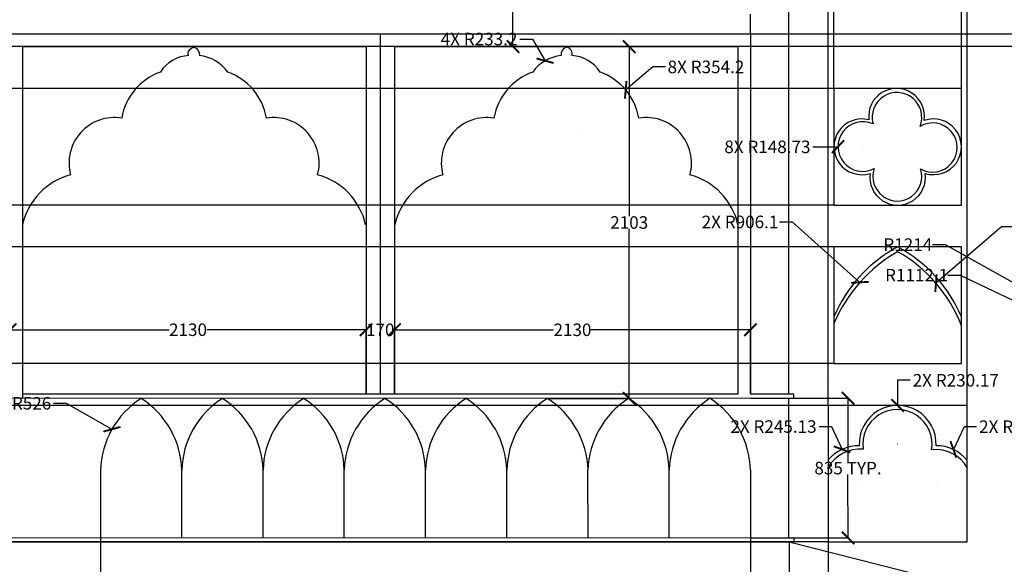
# Model space of a CAD drawing. Units: inches. Extents: x 829 to 33356404, y 1874 to 16983.
# Tile 4 of 9: x 4957 to 10848, y 9032 to 12288. Entities that reach past the tile are written whole.
import ezdxf

# ---------------------------------------------------------------- set-up
doc = ezdxf.new("R2010")
doc.units = ezdxf.units.IN
doc.header["$MEASUREMENT"] = 0
doc.header["$PDMODE"] = 3
doc.layers.add('A-ANNO-DIMS', color=2, linetype='Continuous', lineweight=18)
doc.layers.add('A-ELEV', color=7, linetype='Continuous', lineweight=25)
doc.styles.get("Standard").update_dxf_attribs({"font": 'arial.ttf'})
doc.dimstyles.get("Standard").update_dxf_attribs({"dimtxt": 75, "dimasz": 75, "dimexe": 0.18, "dimexo": 0.0625, "dimgap": 0.09, "dimtad": 0, "dimtih": 1, "dimtoh": 1, "dimdec": 0, "dimzin": 0, "dimdsep": 46, "dimtxsty": 'Standard', "dimblk": 'ARCHTICK', "dimcen": 0.09, "dimadec": 0, "dimazin": 0, "dimtfac": 1, "dimtdec": 0, "dimtofl": 0, "dimtmove": 0, "dimatfit": 3, "dimfxl": 1, "dimtolj": 1, "dimtzin": 0, "dimarcsym": 0})

# ---------------------------------------------------------------- blocks, each defined once
blk = doc.blocks.new('_ArchTick')
at = {"color": 0, "linetype": 'ByBlock', "const_width": 0.15}
blk.add_lwpolyline([(-0.5, -0.5), (0.5, 0.5)], dxfattribs=at)
blk = doc.blocks.new('*D35')
at = {"layer": 'A-ANNO-DIMS', "color": 0, "lineweight": -2, "transparency": 16777216}
for p, q in [((7957.3, 12669.2), (7908.7, 12669.2)), ((7908.8, 12669.2), (7908.8, 12434.2)), ((7908.8, 12127.2), (7908.8, 12357.4)), ((7957.3, 12127.2), (7908.7, 12127.2))]:
    blk.add_line(p, q, dxfattribs=at)
at = {"layer": 'Defpoints', "color": 0, "transparency": 16777216}
for p in [(7908.8, 12669.2), (7957.3, 12669.2), (7957.3, 12127.2)]:
    blk.add_point(p, dxfattribs=at)
at = {"layer": 'A-ANNO-DIMS', "color": 0, "lineweight": -2, "transparency": 16777216, "xscale": 75, "yscale": 75, "zscale": 75}
for p, rotation in [((7908.8, 12669.2), 90), ((7908.8, 12127.2), 270)]:
    blk.add_blockref('_ArchTick', p, dxfattribs=dict(at, rotation=rotation))
at = {"layer": 'A-ANNO-DIMS', "color": 0, "transparency": 16777216, "insert": (7908.8, 12395.8), "char_height": 75, "attachment_point": 5}
blk.add_mtext('\\A1;542', dxfattribs=at)
blk = doc.blocks.new('*D42')
at = {"layer": 'A-ANNO-DIMS', "color": 0, "lineweight": -2, "transparency": 16777216}
for p, q in [((8125.2, 12127.2), (8604.3, 12127.2)), ((8604.2, 12127.2), (8604.2, 11114.1)), ((8604.2, 10024.2), (8604.2, 11037.3)), ((8125.2, 10024.2), (8604.3, 10024.2))]:
    blk.add_line(p, q, dxfattribs=at)
at = {"layer": 'Defpoints', "color": 0, "transparency": 16777216}
for p in [(8125.1, 12127.2), (8604.2, 12127.2), (8125.1, 10024.2)]:
    blk.add_point(p, dxfattribs=at)
at = {"layer": 'A-ANNO-DIMS', "color": 0, "lineweight": -2, "transparency": 16777216, "xscale": 75, "yscale": 75, "zscale": 75}
for p, rotation in [((8604.2, 12127.2), 90), ((8604.2, 10024.2), 270)]:
    blk.add_blockref('_ArchTick', p, dxfattribs=dict(at, rotation=rotation))
at = {"layer": 'A-ANNO-DIMS', "color": 0, "transparency": 16777216, "insert": (8604.2, 11075.7), "char_height": 75, "attachment_point": 5}
blk.add_mtext('\\A1;2103', dxfattribs=at)
blk = doc.blocks.new('*D44')
at = {"layer": 'A-ANNO-DIMS', "color": 0, "lineweight": -2, "transparency": 16777216}
for p, q in [((4899.4, 10049.5), (4899.4, 10434.9)), ((4899.4, 10434.7), (5851.9, 10434.7)), ((7029.7, 10434.7), (6077.1, 10434.7)), ((7029.7, 10049.5), (7029.7, 10434.9))]:
    blk.add_line(p, q, dxfattribs=at)
at = {"layer": 'Defpoints', "color": 0, "transparency": 16777216}
for p in [(4899.4, 10434.7), (4899.4, 10049.4), (7029.7, 10049.4)]:
    blk.add_point(p, dxfattribs=at)
at = {"layer": 'A-ANNO-DIMS', "color": 0, "lineweight": -2, "transparency": 16777216, "xscale": 75, "yscale": 75, "zscale": 75, "rotation": 180}
blk.add_blockref('_ArchTick', (4899.4, 10434.7), dxfattribs=at)
at = {"layer": 'A-ANNO-DIMS', "color": 0, "lineweight": -2, "transparency": 16777216, "xscale": 75, "yscale": 75, "zscale": 75}
blk.add_blockref('_ArchTick', (7029.7, 10434.7), dxfattribs=at)
at = {"layer": 'A-ANNO-DIMS', "color": 0, "transparency": 16777216, "insert": (5964.5, 10434.7), "char_height": 75, "attachment_point": 5}
blk.add_mtext('\\A1;2130', dxfattribs=at)
blk = doc.blocks.new('*D45')
at = {"layer": 'A-ANNO-DIMS', "color": 0, "lineweight": -2, "transparency": 16777216}
for p, q in [((7199.7, 10049.5), (7199.7, 10434.5)), ((7199.7, 10434.3), (8152.1, 10434.3)), ((9329.8, 10434.3), (8377.3, 10434.3)), ((9329.8, 10049.5), (9329.8, 10434.5))]:
    blk.add_line(p, q, dxfattribs=at)
at = {"layer": 'Defpoints', "color": 0, "transparency": 16777216}
for p in [(7199.7, 10434.3), (7199.7, 10049.4), (9329.8, 10049.4)]:
    blk.add_point(p, dxfattribs=at)
at = {"layer": 'A-ANNO-DIMS', "color": 0, "lineweight": -2, "transparency": 16777216, "xscale": 75, "yscale": 75, "zscale": 75, "rotation": 180}
blk.add_blockref('_ArchTick', (7199.7, 10434.3), dxfattribs=at)
at = {"layer": 'A-ANNO-DIMS', "color": 0, "lineweight": -2, "transparency": 16777216, "xscale": 75, "yscale": 75, "zscale": 75}
blk.add_blockref('_ArchTick', (9329.8, 10434.3), dxfattribs=at)
at = {"layer": 'A-ANNO-DIMS', "color": 0, "transparency": 16777216, "insert": (8264.7, 10434.3), "char_height": 75, "attachment_point": 5}
blk.add_mtext('\\A1;2130', dxfattribs=at)
blk = doc.blocks.new('*D43')
at = {"layer": 'A-ANNO-DIMS', "color": 0, "lineweight": -2, "transparency": 16777216}
for p, q in [((7029.7, 10049.5), (7029.7, 10434.5)), ((7029.7, 10434.3), (7035.4, 10434.3)), ((7199.7, 10434.3), (7194, 10434.3)), ((7199.7, 10049.5), (7199.7, 10434.5))]:
    blk.add_line(p, q, dxfattribs=at)
at = {"layer": 'Defpoints', "color": 0, "transparency": 16777216}
for p in [(7029.7, 10434.3), (7029.7, 10049.4), (7199.7, 10049.4)]:
    blk.add_point(p, dxfattribs=at)
at = {"layer": 'A-ANNO-DIMS', "color": 0, "lineweight": -2, "transparency": 16777216, "xscale": 75, "yscale": 75, "zscale": 75, "rotation": 180}
blk.add_blockref('_ArchTick', (7029.7, 10434.3), dxfattribs=at)
at = {"layer": 'A-ANNO-DIMS', "color": 0, "lineweight": -2, "transparency": 16777216, "xscale": 75, "yscale": 75, "zscale": 75}
blk.add_blockref('_ArchTick', (7199.7, 10434.3), dxfattribs=at)
at = {"layer": 'A-ANNO-DIMS', "color": 0, "transparency": 16777216, "insert": (7114.7, 10434.3), "char_height": 75, "attachment_point": 5}
blk.add_mtext('\\A1;170', dxfattribs=at)
blk = doc.blocks.new('ARCADE-ARCHES')
for p, q in [((0.1, 405.5), (0, 0.5)), ((486.1, 0.4), (486.1, 405.4)), ((972.1, 0.4), (972.2, 405.4)), ((1458.2, 0.3), (1458.2, 405.3)), ((1944.3, 0.2), (1944.3, 405.3)), ((2430.3, 0.2), (2430.4, 405.2)), ((2916.4, 0.1), (2916.4, 405.2)), ((3402.4, 0.1), (3402.5, 405.1)), ((3888.7, 405.2), (3888.7, 0))]:
    blk.add_line(p, q)
for centre, start, end in [((525.9, 391.9), 122.51468, 178.52248), ((-39.6, 391.9), 1.47752, 57.48532), ((1011.9, 391.9), 122.51468, 178.52248), ((446.5, 391.9), 1.47752, 57.48532), ((1498, 391.9), 122.51468, 178.52248), ((932.6, 391.9), 1.47752, 57.48532), ((1984.2, 391.9), 122.51468, 178.52248), ((1418.7, 391.9), 1.47752, 57.48532), ((2470.1, 391.7), 122.51468, 178.52248), ((1904.7, 391.7), 1.47752, 57.48532), ((2956.2, 391.7), 122.51468, 178.52248), ((2390.7, 391.7), 1.47752, 57.48532), ((3442.2, 391.6), 122.51468, 178.52248), ((2876.8, 391.6), 1.47752, 57.48532), ((3928.4, 391.6), 122.51468, 178.52248), ((3362.9, 391.6), 1.47752, 57.48532)]:
    blk.add_arc(centre, 526, start, end)
blk = doc.blocks.new('*D80')
at = {"layer": 'A-ANNO-DIMS', "color": 0, "lineweight": -2, "transparency": 16777216}
for p, q in [((5441.3, 9188.4), (5441.4, 8604.9)), ((9330, 9189.3), (9330.2, 8605.9)), ((5441.4, 8605.1), (6677, 8605.4)), ((9330.2, 8606.1), (8094.6, 8605.8))]:
    blk.add_line(p, q, dxfattribs=at)
at = {"layer": 'Defpoints', "color": 0, "transparency": 16777216}
for p in [(5441.3, 9188.4), (9330, 9189.4), (9330.2, 8606.1)]:
    blk.add_point(p, dxfattribs=at)
at = {"layer": 'A-ANNO-DIMS', "color": 0, "lineweight": -2, "transparency": 16777216, "xscale": 75, "yscale": 75, "zscale": 75}
for p, rotation in [((5441.4, 8605.1), 180.0138445878549), ((9330.2, 8606.1), 0.0138445878549074)]:
    blk.add_blockref('_ArchTick', p, dxfattribs=dict(at, rotation=rotation))
at = {"layer": 'A-ANNO-DIMS', "color": 0, "transparency": 16777216, "insert": (7385.8, 8605.6), "char_height": 75, "attachment_point": 5}
blk.add_mtext('\\A1;ARCADE ARCHES 3889 TYP.', dxfattribs=at)
blk = doc.blocks.new('*D81')
at = {"layer": 'A-ANNO-DIMS', "color": 0, "lineweight": -2, "transparency": 16777216}
for p, q in [((9329.9, 10024.8), (9913.3, 10025)), ((9913.1, 10025), (9913.2, 9645.7)), ((9913.3, 9189.5), (9913.2, 9568.8)), ((9330.1, 9189.4), (9913.5, 9189.5))]:
    blk.add_line(p, q, dxfattribs=at)
at = {"layer": 'Defpoints', "color": 0, "transparency": 16777216}
for p in [(9329.8, 10024.8), (9913.1, 10025), (9330, 9189.4)]:
    blk.add_point(p, dxfattribs=at)
at = {"layer": 'A-ANNO-DIMS', "color": 0, "lineweight": -2, "transparency": 16777216, "xscale": 75, "yscale": 75, "zscale": 75}
for p, rotation in [((9913.1, 10025), 90.01384458785488), ((9913.3, 9189.5), 270.0138445878549)]:
    blk.add_blockref('_ArchTick', p, dxfattribs=dict(at, rotation=rotation))
at = {"layer": 'A-ANNO-DIMS', "color": 0, "transparency": 16777216, "insert": (9913.2, 9607.2), "char_height": 75, "attachment_point": 5}
blk.add_mtext('\\A1;835 TYP.', dxfattribs=at)
blk = doc.blocks.new('*D83')
at = {"layer": 'A-ANNO-DIMS', "color": 0, "lineweight": -2, "transparency": 16777216}
for p, q in [((13604.5, 15734.9), (985.4, 15734.9)), ((985.6, 15734.9), (985.6, 10279.1)), ((985.6, 4746.5), (985.6, 10202.3)), ((3169.7, 4746.5), (985.4, 4746.5))]:
    blk.add_line(p, q, dxfattribs=at)
at = {"layer": 'Defpoints', "color": 0, "transparency": 16777216}
for p in [(985.6, 15734.9), (13604.5, 15734.9), (3169.8, 4746.5)]:
    blk.add_point(p, dxfattribs=at)
at = {"layer": 'A-ANNO-DIMS', "color": 0, "lineweight": -2, "transparency": 16777216, "xscale": 75, "yscale": 75, "zscale": 75}
for p, rotation in [((985.6, 15734.9), 90), ((985.6, 4746.5), 270)]:
    blk.add_blockref('_ArchTick', p, dxfattribs=dict(at, rotation=rotation))
at = {"layer": 'A-ANNO-DIMS', "color": 0, "transparency": 16777216, "insert": (985.6, 10240.7), "char_height": 75, "attachment_point": 5}
blk.add_mtext('\\A1;10988', dxfattribs=at)
blk = doc.blocks.new('*D98')
at = {"layer": 'A-ANNO-DIMS', "color": 0, "lineweight": -2, "transparency": 16777216}
for p, q in [((9793.7, 9165.5), (985.4, 9165.5)), ((985.6, 9165.5), (985.6, 9057.4)), ((985.6, 8872.5), (985.6, 8980.6)), ((9793.7, 8872.5), (985.4, 8872.5))]:
    blk.add_line(p, q, dxfattribs=at)
at = {"layer": 'Defpoints', "color": 0, "transparency": 16777216}
for p in [(985.6, 9165.5), (9793.7, 9165.5), (9793.7, 8872.5)]:
    blk.add_point(p, dxfattribs=at)
at = {"layer": 'A-ANNO-DIMS', "color": 0, "lineweight": -2, "transparency": 16777216, "xscale": 75, "yscale": 75, "zscale": 75}
for p, rotation in [((985.6, 9165.5), 90), ((985.6, 8872.5), 270)]:
    blk.add_blockref('_ArchTick', p, dxfattribs=dict(at, rotation=rotation))
at = {"layer": 'A-ANNO-DIMS', "color": 0, "transparency": 16777216, "insert": (985.6, 9019), "char_height": 75, "attachment_point": 5}
blk.add_mtext('\\A1;293', dxfattribs=at)
blk = doc.blocks.new('*D99')
at = {"layer": 'A-ANNO-DIMS', "color": 0, "lineweight": -2, "transparency": 16777216}
for p, q in [((9793.7, 9982.2), (985.4, 9982.2)), ((985.6, 9982.2), (985.6, 9612.2)), ((985.6, 9165.5), (985.6, 9535.4)), ((9793.7, 9165.5), (985.4, 9165.5))]:
    blk.add_line(p, q, dxfattribs=at)
at = {"layer": 'Defpoints', "color": 0, "transparency": 16777216}
for p in [(985.6, 9982.2), (9793.7, 9982.2), (9793.7, 9165.5)]:
    blk.add_point(p, dxfattribs=at)
at = {"layer": 'A-ANNO-DIMS', "color": 0, "lineweight": -2, "transparency": 16777216, "xscale": 75, "yscale": 75, "zscale": 75}
for p, rotation in [((985.6, 9982.2), 90), ((985.6, 9165.5), 270)]:
    blk.add_blockref('_ArchTick', p, dxfattribs=dict(at, rotation=rotation))
at = {"layer": 'A-ANNO-DIMS', "color": 0, "transparency": 16777216, "insert": (985.6, 9573.8), "char_height": 75, "attachment_point": 5}
blk.add_mtext('\\A1;816.7', dxfattribs=at)
blk = doc.blocks.new('*D100')
at = {"layer": 'A-ANNO-DIMS', "color": 0, "lineweight": -2, "transparency": 16777216}
for p, q in [((9829.1, 10232.2), (985.4, 10232.2)), ((985.6, 10232.2), (985.6, 10145.6)), ((985.6, 9982.2), (985.6, 10068.8)), ((9793.7, 9982.2), (985.4, 9982.2))]:
    blk.add_line(p, q, dxfattribs=at)
at = {"layer": 'Defpoints', "color": 0, "transparency": 16777216}
for p in [(985.6, 10232.2), (9829.2, 10232.2), (9793.7, 9982.2)]:
    blk.add_point(p, dxfattribs=at)
at = {"layer": 'A-ANNO-DIMS', "color": 0, "lineweight": -2, "transparency": 16777216, "xscale": 75, "yscale": 75, "zscale": 75}
for p, rotation in [((985.6, 10232.2), 90), ((985.6, 9982.2), 270)]:
    blk.add_blockref('_ArchTick', p, dxfattribs=dict(at, rotation=rotation))
at = {"layer": 'A-ANNO-DIMS', "color": 0, "transparency": 16777216, "insert": (985.6, 10107.2), "char_height": 75, "attachment_point": 5}
blk.add_mtext('\\A1;250', dxfattribs=at)
blk = doc.blocks.new('*D101')
at = {"layer": 'A-ANNO-DIMS', "color": 0, "lineweight": -2, "transparency": 16777216}
for p, q in [((9829.1, 10929.7), (985.4, 10929.7)), ((985.6, 10929.7), (985.6, 10619.3)), ((985.6, 10232.2), (985.6, 10542.6)), ((9829.1, 10232.2), (985.4, 10232.2))]:
    blk.add_line(p, q, dxfattribs=at)
at = {"layer": 'Defpoints', "color": 0, "transparency": 16777216}
for p in [(985.6, 10929.7), (9829.2, 10929.7), (9829.2, 10232.2)]:
    blk.add_point(p, dxfattribs=at)
at = {"layer": 'A-ANNO-DIMS', "color": 0, "lineweight": -2, "transparency": 16777216, "xscale": 75, "yscale": 75, "zscale": 75}
for p, rotation in [((985.6, 10929.7), 90), ((985.6, 10232.2), 270)]:
    blk.add_blockref('_ArchTick', p, dxfattribs=dict(at, rotation=rotation))
at = {"layer": 'A-ANNO-DIMS', "color": 0, "transparency": 16777216, "insert": (985.6, 10580.9), "char_height": 75, "attachment_point": 5}
blk.add_mtext('\\A1;697.5', dxfattribs=at)
blk = doc.blocks.new('*D102')
at = {"layer": 'A-ANNO-DIMS', "color": 0, "lineweight": -2, "transparency": 16777216}
for p, q in [((9829.1, 11179.7), (985.4, 11179.7)), ((985.6, 11179.7), (985.6, 11093.1)), ((985.6, 10929.7), (985.6, 11016.3)), ((9829.1, 10929.7), (985.4, 10929.7))]:
    blk.add_line(p, q, dxfattribs=at)
at = {"layer": 'Defpoints', "color": 0, "transparency": 16777216}
for p in [(985.6, 11179.7), (9829.2, 11179.7), (9829.2, 10929.7)]:
    blk.add_point(p, dxfattribs=at)
at = {"layer": 'A-ANNO-DIMS', "color": 0, "lineweight": -2, "transparency": 16777216, "xscale": 75, "yscale": 75, "zscale": 75}
for p, rotation in [((985.6, 11179.7), 90), ((985.6, 10929.7), 270)]:
    blk.add_blockref('_ArchTick', p, dxfattribs=dict(at, rotation=rotation))
at = {"layer": 'A-ANNO-DIMS', "color": 0, "transparency": 16777216, "insert": (985.6, 11054.7), "char_height": 75, "attachment_point": 5}
blk.add_mtext('\\A1;250', dxfattribs=at)
blk = doc.blocks.new('*D103')
at = {"layer": 'A-ANNO-DIMS', "color": 0, "lineweight": -2, "transparency": 16777216}
for p, q in [((9829.1, 11877.2), (985.4, 11877.2)), ((985.6, 11877.2), (985.6, 11566.8)), ((985.6, 11179.7), (985.6, 11490.1)), ((9829.1, 11179.7), (985.4, 11179.7))]:
    blk.add_line(p, q, dxfattribs=at)
at = {"layer": 'Defpoints', "color": 0, "transparency": 16777216}
for p in [(985.6, 11877.2), (9829.2, 11877.2), (9829.2, 11179.7)]:
    blk.add_point(p, dxfattribs=at)
at = {"layer": 'A-ANNO-DIMS', "color": 0, "lineweight": -2, "transparency": 16777216, "xscale": 75, "yscale": 75, "zscale": 75}
for p, rotation in [((985.6, 11877.2), 90), ((985.6, 11179.7), 270)]:
    blk.add_blockref('_ArchTick', p, dxfattribs=dict(at, rotation=rotation))
at = {"layer": 'A-ANNO-DIMS', "color": 0, "transparency": 16777216, "insert": (985.6, 11528.5), "char_height": 75, "attachment_point": 5}
blk.add_mtext('\\A1;697.5', dxfattribs=at)
blk = doc.blocks.new('*D104')
at = {"layer": 'A-ANNO-DIMS', "color": 0, "lineweight": -2, "transparency": 16777216}
for p, q in [((9559.8, 12127.2), (985.4, 12127.2)), ((985.6, 12127.2), (985.6, 12040.6)), ((985.6, 11877.2), (985.6, 11963.8)), ((9829.1, 11877.2), (985.4, 11877.2))]:
    blk.add_line(p, q, dxfattribs=at)
at = {"layer": 'Defpoints', "color": 0, "transparency": 16777216}
for p in [(985.6, 12127.2), (9559.8, 12127.2), (9829.2, 11877.2)]:
    blk.add_point(p, dxfattribs=at)
at = {"layer": 'A-ANNO-DIMS', "color": 0, "lineweight": -2, "transparency": 16777216, "xscale": 75, "yscale": 75, "zscale": 75}
for p, rotation in [((985.6, 12127.2), 90), ((985.6, 11877.2), 270)]:
    blk.add_blockref('_ArchTick', p, dxfattribs=dict(at, rotation=rotation))
at = {"layer": 'A-ANNO-DIMS', "color": 0, "transparency": 16777216, "insert": (985.6, 12002.2), "char_height": 75, "attachment_point": 5}
blk.add_mtext('\\A1;250', dxfattribs=at)
blk = doc.blocks.new('*D105')
at = {"layer": 'A-ANNO-DIMS', "color": 0, "lineweight": -2, "transparency": 16777216}
for p, q in [((9829.2, 11877.3), (9829.2, 16934.2)), ((9829.2, 16934), (10084, 16934)), ((10591.5, 16934), (10336.6, 16934)), ((10591.5, 11877.3), (10591.5, 16934.2))]:
    blk.add_line(p, q, dxfattribs=at)
at = {"layer": 'Defpoints', "color": 0, "transparency": 16777216}
for p in [(10591.5, 16934), (9829.2, 11877.2), (10591.5, 11877.2)]:
    blk.add_point(p, dxfattribs=at)
at = {"layer": 'A-ANNO-DIMS', "color": 0, "lineweight": -2, "transparency": 16777216, "xscale": 75, "yscale": 75, "zscale": 75, "rotation": 180}
blk.add_blockref('_ArchTick', (9829.2, 16934), dxfattribs=at)
at = {"layer": 'A-ANNO-DIMS', "color": 0, "lineweight": -2, "transparency": 16777216, "xscale": 75, "yscale": 75, "zscale": 75}
blk.add_blockref('_ArchTick', (10591.5, 16934), dxfattribs=at)
at = {"layer": 'A-ANNO-DIMS', "color": 0, "transparency": 16777216, "insert": (10210.3, 16934), "char_height": 75, "attachment_point": 5}
blk.add_mtext('\\A1;762.3', dxfattribs=at)
blk = doc.blocks.new('*D106')
at = {"layer": 'A-ANNO-DIMS', "color": 0, "lineweight": -2, "transparency": 16777216}
for p, q in [((9559.8, 12127.3), (9559.8, 16934.2)), ((9559.8, 16934), (9567.2, 16934)), ((9829.2, 16934), (9821.8, 16934)), ((9829.2, 11877.3), (9829.2, 16934.2))]:
    blk.add_line(p, q, dxfattribs=at)
at = {"layer": 'Defpoints', "color": 0, "transparency": 16777216}
for p in [(9829.2, 16934), (9559.8, 12127.2), (9829.2, 11877.2)]:
    blk.add_point(p, dxfattribs=at)
at = {"layer": 'A-ANNO-DIMS', "color": 0, "lineweight": -2, "transparency": 16777216, "xscale": 75, "yscale": 75, "zscale": 75, "rotation": 180}
blk.add_blockref('_ArchTick', (9559.8, 16934), dxfattribs=at)
at = {"layer": 'A-ANNO-DIMS', "color": 0, "lineweight": -2, "transparency": 16777216, "xscale": 75, "yscale": 75, "zscale": 75}
blk.add_blockref('_ArchTick', (9829.2, 16934), dxfattribs=at)
at = {"layer": 'A-ANNO-DIMS', "color": 0, "transparency": 16777216, "insert": (9694.5, 16934), "char_height": 75, "attachment_point": 5}
blk.add_mtext('\\A1;269.3', dxfattribs=at)
blk = doc.blocks.new('*D107')
at = {"layer": 'A-ANNO-DIMS', "color": 0, "lineweight": -2, "transparency": 16777216}
for p, q in [((9793.7, 9982.3), (9793.7, 16934.2)), ((9793.7, 16934), (10084, 16934)), ((10626.9, 16934), (10336.6, 16934)), ((10626.9, 9982.3), (10626.9, 16934.2))]:
    blk.add_line(p, q, dxfattribs=at)
at = {"layer": 'Defpoints', "color": 0, "transparency": 16777216}
for p in [(10626.9, 16934), (9793.7, 9982.2), (10626.9, 9982.2)]:
    blk.add_point(p, dxfattribs=at)
at = {"layer": 'A-ANNO-DIMS', "color": 0, "lineweight": -2, "transparency": 16777216, "xscale": 75, "yscale": 75, "zscale": 75, "rotation": 180}
blk.add_blockref('_ArchTick', (9793.7, 16934), dxfattribs=at)
at = {"layer": 'A-ANNO-DIMS', "color": 0, "lineweight": -2, "transparency": 16777216, "xscale": 75, "yscale": 75, "zscale": 75}
blk.add_blockref('_ArchTick', (10626.9, 16934), dxfattribs=at)
at = {"layer": 'A-ANNO-DIMS', "color": 0, "transparency": 16777216, "insert": (10210.3, 16934), "char_height": 75, "attachment_point": 5}
blk.add_mtext('\\A1;833.2', dxfattribs=at)
blk = doc.blocks.new('*D108')
at = {"layer": 'A-ANNO-DIMS', "color": 0, "lineweight": -2, "transparency": 16777216}
for p, q in [((9560.3, 9165.4), (9560.3, 3551.3)), ((9793.7, 9165.4), (9793.7, 3551.3)), ((9560.3, 3551.5), (9793.7, 3551.5)), ((9793.7, 3551.5), (9868.7, 3551.5))]:
    blk.add_line(p, q, dxfattribs=at)
at = {"layer": 'Defpoints', "color": 0, "transparency": 16777216}
for p in [(9560.3, 9165.5), (9793.7, 9165.5), (9793.7, 3551.5)]:
    blk.add_point(p, dxfattribs=at)
at = {"layer": 'A-ANNO-DIMS', "color": 0, "lineweight": -2, "transparency": 16777216, "xscale": 75, "yscale": 75, "zscale": 75, "rotation": 180}
blk.add_blockref('_ArchTick', (9560.3, 3551.5), dxfattribs=at)
at = {"layer": 'A-ANNO-DIMS', "color": 0, "lineweight": -2, "transparency": 16777216, "xscale": 75, "yscale": 75, "zscale": 75}
blk.add_blockref('_ArchTick', (9793.7, 3551.5), dxfattribs=at)
at = {"layer": 'A-ANNO-DIMS', "color": 0, "transparency": 16777216, "insert": (9995.8, 3551.5), "char_height": 75, "attachment_point": 5}
blk.add_mtext('\\A1;233.4', dxfattribs=at)
blk = doc.blocks.new('*D111')
at = {"layer": 'A-ANNO-DIMS', "color": 0, "lineweight": -2, "transparency": 16777216}
for p, q in [((8745.5, 12006), (8583.1, 11869)), ((8820.5, 12006), (8745.5, 12006)), ((8312.3, 11640.6), (8312.3, 11640.7)), ((8312.3, 11640.6), (8312.4, 11640.6))]:
    blk.add_line(p, q, dxfattribs=at)
at = {"layer": 'Defpoints', "color": 0, "transparency": 16777216}
for p in [(8583.1, 11869), (8312.3, 11640.6)]:
    blk.add_point(p, dxfattribs=at)
at = {"layer": 'A-ANNO-DIMS', "color": 0, "lineweight": -2, "transparency": 16777216, "xscale": 75, "yscale": 75, "zscale": 75, "rotation": 220.1417111972914}
blk.add_blockref('_ArchTick', (8583.1, 11869), dxfattribs=at)
at = {"layer": 'A-ANNO-DIMS', "color": 0, "transparency": 16777216, "insert": (9063.3, 12006), "char_height": 75, "attachment_point": 5}
blk.add_mtext('\\A1;8X R354.2', dxfattribs=at)
blk = doc.blocks.new('*D113')
at = {"layer": 'A-ANNO-DIMS', "color": 0, "lineweight": -2, "transparency": 16777216}
for p, q in [((7950.2, 12172.5), (8025.2, 12172.5)), ((8025.2, 12172.5), (8100.6, 12042.8)), ((8217.8, 11841.2), (8218, 11841.2)), ((8217.9, 11841.2), (8217.9, 11841.3))]:
    blk.add_line(p, q, dxfattribs=at)
at = {"layer": 'Defpoints', "color": 0, "transparency": 16777216}
for p in [(8100.6, 12042.8), (8217.9, 11841.2)]:
    blk.add_point(p, dxfattribs=at)
at = {"layer": 'A-ANNO-DIMS', "color": 0, "lineweight": -2, "transparency": 16777216, "xscale": 75, "yscale": 75, "zscale": 75, "rotation": 300.1902752682242}
blk.add_blockref('_ArchTick', (8100.6, 12042.8), dxfattribs=at)
at = {"layer": 'A-ANNO-DIMS', "color": 0, "transparency": 16777216, "insert": (7705.9, 12172.5), "char_height": 75, "attachment_point": 5}
blk.add_mtext('\\A1;4X R233.2', dxfattribs=at)
blk = doc.blocks.new('*D114')
at = {"layer": 'A-ANNO-DIMS', "color": 0, "lineweight": -2, "transparency": 16777216}
for p, q in [((5159.5, 9994.8), (5234.5, 9994.8)), ((5234.5, 9994.8), (5509.2, 9839.5)), ((5967, 9580.4), (5967, 9580.6)), ((5967, 9580.5), (5967.1, 9580.5))]:
    blk.add_line(p, q, dxfattribs=at)
at = {"layer": 'Defpoints', "color": 0, "transparency": 16777216}
for p in [(5509.2, 9839.5), (5967, 9580.5)]:
    blk.add_point(p, dxfattribs=at)
at = {"layer": 'A-ANNO-DIMS', "color": 0, "lineweight": -2, "transparency": 16777216, "xscale": 75, "yscale": 75, "zscale": 75, "rotation": 330.5044086003726}
blk.add_blockref('_ArchTick', (5509.2, 9839.5), dxfattribs=at)
at = {"layer": 'A-ANNO-DIMS', "color": 0, "transparency": 16777216, "insert": (4931.1, 9994.8), "char_height": 75, "attachment_point": 5}
blk.add_mtext('\\A1;32X R526', dxfattribs=at)
blk = doc.blocks.new('*D123')
at = {"layer": 'A-ANNO-DIMS', "color": 0, "lineweight": -2, "transparency": 16777216}
for p, q in [((10418.6, 10943.5), (10493.6, 10943.5)), ((10493.6, 10943.5), (11130.3, 10589.5)), ((12191.3, 9999.5), (12191.5, 9999.5)), ((12191.4, 9999.4), (12191.4, 9999.6))]:
    blk.add_line(p, q, dxfattribs=at)
at = {"layer": 'Defpoints', "color": 0, "transparency": 16777216}
for p in [(11130.3, 10589.5), (12191.4, 9999.5)]:
    blk.add_point(p, dxfattribs=at)
at = {"layer": 'A-ANNO-DIMS', "color": 0, "lineweight": -2, "transparency": 16777216, "xscale": 75, "yscale": 75, "zscale": 75, "rotation": 330.9254937916661}
blk.add_blockref('_ArchTick', (11130.3, 10589.5), dxfattribs=at)
at = {"layer": 'A-ANNO-DIMS', "color": 0, "transparency": 16777216, "insert": (10270.8, 10943.5), "char_height": 75, "attachment_point": 5}
blk.add_mtext('\\A1;R1214', dxfattribs=at)
blk = doc.blocks.new('*D124')
at = {"layer": 'A-ANNO-DIMS', "color": 0, "lineweight": -2, "transparency": 16777216}
for p, q in [((10508.3, 10761.1), (10583.3, 10761.1)), ((10583.3, 10761.1), (11186.3, 10475.5)), ((12191.3, 9999.5), (12191.5, 9999.5)), ((12191.4, 9999.4), (12191.4, 9999.6))]:
    blk.add_line(p, q, dxfattribs=at)
at = {"layer": 'Defpoints', "color": 0, "transparency": 16777216}
for p in [(11186.3, 10475.5), (12191.4, 9999.5)]:
    blk.add_point(p, dxfattribs=at)
at = {"layer": 'A-ANNO-DIMS', "color": 0, "lineweight": -2, "transparency": 16777216, "xscale": 75, "yscale": 75, "zscale": 75, "rotation": 334.6586083454434}
blk.add_blockref('_ArchTick', (11186.3, 10475.5), dxfattribs=at)
at = {"layer": 'A-ANNO-DIMS', "color": 0, "transparency": 16777216, "insert": (10323.9, 10761.1), "char_height": 75, "attachment_point": 5}
blk.add_mtext('\\A1;R1112.1', dxfattribs=at)
blk = doc.blocks.new('*D128')
at = {"layer": 'A-ANNO-DIMS', "color": 0, "lineweight": -2, "transparency": 16777216}
for p, q in [((9503.7, 11079.2), (9578.7, 11079.2)), ((9578.7, 11079.2), (9984.9, 10717.9)), ((10661.9, 10115.8), (10662.1, 10115.8)), ((10662, 10115.7), (10662, 10115.8))]:
    blk.add_line(p, q, dxfattribs=at)
at = {"layer": 'Defpoints', "color": 0, "transparency": 16777216}
for p in [(9984.9, 10717.9), (10662, 10115.8)]:
    blk.add_point(p, dxfattribs=at)
at = {"layer": 'A-ANNO-DIMS', "color": 0, "lineweight": -2, "transparency": 16777216, "xscale": 75, "yscale": 75, "zscale": 75, "rotation": 318.3509099254765}
blk.add_blockref('_ArchTick', (9984.9, 10717.9), dxfattribs=at)
at = {"layer": 'A-ANNO-DIMS', "color": 0, "transparency": 16777216, "insert": (9267.2, 11079.2), "char_height": 75, "attachment_point": 5}
blk.add_mtext('\\A1;2X R906.1', dxfattribs=at)
blk = doc.blocks.new('*D129')
at = {"layer": 'A-ANNO-DIMS', "color": 0, "lineweight": -2, "transparency": 16777216}
for p, q in [((10830.9, 11050.5), (10439.6, 10713.3)), ((10905.9, 11050.5), (10830.9, 11050.5)), ((9787.3, 10151.5), (9787.5, 10151.5)), ((9787.4, 10151.4), (9787.4, 10151.6))]:
    blk.add_line(p, q, dxfattribs=at)
at = {"layer": 'Defpoints', "color": 0, "transparency": 16777216}
for p in [(10439.6, 10713.3), (9787.4, 10151.5)]:
    blk.add_point(p, dxfattribs=at)
at = {"layer": 'A-ANNO-DIMS', "color": 0, "lineweight": -2, "transparency": 16777216, "xscale": 75, "yscale": 75, "zscale": 75, "rotation": 220.7456490042762}
blk.add_blockref('_ArchTick', (10439.6, 10713.3), dxfattribs=at)
at = {"layer": 'A-ANNO-DIMS', "color": 0, "transparency": 16777216, "insert": (11149.7, 11050.5), "char_height": 75, "attachment_point": 5}
blk.add_mtext('\\A1;2X R860.8', dxfattribs=at)
blk = doc.blocks.new('*D133')
at = {"layer": 'A-ANNO-DIMS', "color": 0, "lineweight": -2, "transparency": 16777216}
for p, q in [((9740.4, 9855.6), (9815.4, 9855.6)), ((9815.4, 9855.6), (9877.7, 9719.1)), ((9979.5, 9496.2), (9979.6, 9496.2)), ((9979.6, 9496.1), (9979.6, 9496.2))]:
    blk.add_line(p, q, dxfattribs=at)
at = {"layer": 'Defpoints', "color": 0, "transparency": 16777216}
for p in [(9877.7, 9719.1), (9979.6, 9496.2)]:
    blk.add_point(p, dxfattribs=at)
at = {"layer": 'A-ANNO-DIMS', "color": 0, "lineweight": -2, "transparency": 16777216, "xscale": 75, "yscale": 75, "zscale": 75, "rotation": 294.5471256031039}
blk.add_blockref('_ArchTick', (9877.7, 9719.1), dxfattribs=at)
at = {"layer": 'A-ANNO-DIMS', "color": 0, "transparency": 16777216, "insert": (9467.5, 9855.6), "char_height": 75, "attachment_point": 5}
blk.add_mtext('\\A1;2X R245.13', dxfattribs=at)
blk = doc.blocks.new('*D134')
at = {"layer": 'A-ANNO-DIMS', "color": 0, "lineweight": -2, "transparency": 16777216}
for p, q in [((10607.7, 9854.8), (10543.8, 9719.1)), ((10682.7, 9854.8), (10607.7, 9854.8)), ((10444.4, 9508.1), (10444.5, 9508.1)), ((10444.5, 9508), (10444.5, 9508.2))]:
    blk.add_line(p, q, dxfattribs=at)
at = {"layer": 'Defpoints', "color": 0, "transparency": 16777216}
for p in [(10543.8, 9719.1), (10444.5, 9508.1)]:
    blk.add_point(p, dxfattribs=at)
at = {"layer": 'A-ANNO-DIMS', "color": 0, "lineweight": -2, "transparency": 16777216, "xscale": 75, "yscale": 75, "zscale": 75, "rotation": 244.7886305373675}
blk.add_blockref('_ArchTick', (10543.8, 9719.1), dxfattribs=at)
at = {"layer": 'A-ANNO-DIMS', "color": 0, "transparency": 16777216, "insert": (10955.6, 9854.8), "char_height": 75, "attachment_point": 5}
blk.add_mtext('\\A1;2X R233.26', dxfattribs=at)
blk = doc.blocks.new('*D135')
at = {"layer": 'A-ANNO-DIMS', "color": 0, "lineweight": -2, "transparency": 16777216}
for p, q in [((10285.3, 10132.2), (10210.3, 10132.2)), ((10210.3, 10132.2), (10210.3, 9982.2)), ((10210.2, 9752.1), (10210.4, 9752.1)), ((10210.3, 9752), (10210.3, 9752.2))]:
    blk.add_line(p, q, dxfattribs=at)
at = {"layer": 'Defpoints', "color": 0, "transparency": 16777216}
for p in [(10210.3, 9982.2), (10210.3, 9752.1)]:
    blk.add_point(p, dxfattribs=at)
at = {"layer": 'A-ANNO-DIMS', "color": 0, "lineweight": -2, "transparency": 16777216, "xscale": 75, "yscale": 75, "zscale": 75, "rotation": 269.999922582549}
blk.add_blockref('_ArchTick', (10210.3, 9982.2), dxfattribs=at)
at = {"layer": 'A-ANNO-DIMS', "color": 0, "transparency": 16777216, "insert": (10558.2, 10132.2), "char_height": 75, "attachment_point": 5}
blk.add_mtext('\\A1;2X R230.17', dxfattribs=at)
blk = doc.blocks.new('*D138')
at = {"layer": 'A-ANNO-DIMS', "color": 0, "lineweight": -2, "transparency": 16777216}
for p, q in [((9703.4, 11528), (9853.4, 11529.1)), ((10002, 11530.1), (10002.2, 11530.1)), ((10002.1, 11530), (10002.1, 11530.2))]:
    blk.add_line(p, q, dxfattribs=at)
at = {"layer": 'Defpoints', "color": 0, "transparency": 16777216}
for p in [(9853.4, 11529.1), (10002.1, 11530.1)]:
    blk.add_point(p, dxfattribs=at)
at = {"layer": 'A-ANNO-DIMS', "color": 0, "lineweight": -2, "transparency": 16777216, "xscale": 75, "yscale": 75, "zscale": 75, "rotation": 0.3944115039448568}
blk.add_blockref('_ArchTick', (9853.4, 11529.1), dxfattribs=at)
at = {"layer": 'A-ANNO-DIMS', "color": 0, "transparency": 16777216, "insert": (9431.1, 11528), "char_height": 75, "attachment_point": 5}
blk.add_mtext('\\A1;8X R148.73', dxfattribs=at)

msp = doc.modelspace()

# ---------------------------------------------------------------- linework, layer by layer
at = {"layer": 'A-ELEV'}
for p, q in [((9329.778, 12202.212), (9329.778, 12320.882)), ((22522.278, 12202.212), (3169.778, 12202.212)), ((7114.404, 12202.212), (7114.669, 10049.392)), ((9329.778, 12202.212), (9329.778, 10049.392)), ((4974.778, 12127.212), (4974.778, 10023.842)), ((4974.778, 12127.212), (7029.666, 12127.212)), ((7029.666, 12127.212), (7029.666, 10049.392)), ((7199.666, 12127.212), (7199.666, 10049.392)), ((7199.666, 12127.212), (9254.778, 12127.212)), ((9254.778, 12127.212), (9254.778, 10049.392)), ((9559.778, 10049.392), (9559.778, 12127.212)), ((18091.883, 12127.212), (9559.826, 12127.212)), ((9589.325, 10024.454), (4899.383, 10023.833)), ((9254.778, 10049.392), (4974.666, 10049.392)), ((9589.325, 10049.392), (9329.778, 10049.392)), ((9559.778, 9189.453), (9559.778, 10024.45)), ((9589.325, 10024.454), (9589.325, 10049.392)), ((3169.778, 9165.468), (9589.325, 9165.468)), ((9589.325, 9189.457), (4872.423, 9188.874)), ((4872.426, 9165.468), (9589.325, 9165.468)), ((9560.336, 9165.468), (10626.905, 8897.385)), ((9589.325, 9189.457), (9589.325, 9165.468))]:
    msp.add_line(p, q, dxfattribs=at)
for points in [[(5966.38, 12073.468, -0.44292011), (6000.762, 12123.624, -0.36773788), (6032.702, 12073.468, -0.24748835)], [(8262.697, 12073.468, 0.44292011), (8228.315, 12123.624, 0.36773788), (8196.374, 12073.468, 0.24748835)]]:
    msp.add_lwpolyline(points, format="xyb", dxfattribs=at)
for points in [[(10591.482, 11877.212), (9829.151, 11877.212), (9829.151, 11179.704), (10591.482, 11179.704)], [(10591.482, 10929.704), (9829.151, 10929.704), (9829.151, 10232.196), (10591.482, 10232.196)], [(10626.905, 9982.196), (9793.728, 9982.196), (9793.728, 9165.468), (10626.905, 9165.468)]]:
    msp.add_lwpolyline(points, close=True, dxfattribs=at)
for centre, radius, start, end in [((5976.392, 11865.187), 208.419, 92.0817943, 148.2984828), ((6011.203, 11841.246), 233.215, 34.9091215, 84.7106013), ((8217.874, 11841.246), 233.215, 95.2893987, 145.0908785), ((8252.685, 11865.187), 208.419, 31.7015172, 87.9182057), ((5916.734, 11640.647), 354.179, 109.4034394, 170.3116953), ((6084.789, 11640.647), 354.179, 9.6883047, 70.5965606), ((8144.288, 11640.647), 354.179, 109.4034394, 170.3116953), ((8312.343, 11640.647), 354.179, 9.6883047, 70.5965606), ((10203.56, 11710.622), 166.726, 351.2838065, 187.1963448), ((10206.216, 11704.536), 148.406, 338.2494566, 195.1245951), ((5525.223, 11430.806), 272.758, 81.0607154, 194.8907352), ((6476.3, 11430.806), 272.758, 345.1092648, 98.9392846), ((7752.776, 11430.806), 272.758, 81.0607154, 194.8907352), ((8703.854, 11430.806), 272.758, 345.1092648, 98.9392846), ((9995.878, 11528.458), 166.726, 75.3135337, 287.1891398), ((10002.136, 11530.089), 148.727, 65.8644078, 297.1118841), ((10419.987, 11523.821), 146.871, 240.147327, 121.1301002), ((10424.756, 11528.458), 166.726, 252.8108602, 109.7700999), ((10208.184, 11350.379), 146.143, 161.1054929, 18.3710533), ((5362.242, 10976.551), 397.12, 104.6768994, 167.65861), ((6639.281, 10976.551), 397.12, 12.34139, 75.3231006), ((7589.796, 10976.551), 397.12, 104.6768994, 167.65861), ((8866.835, 10976.551), 397.12, 12.34139, 75.3231006), ((10210.317, 11346.43), 166.726, 172.1579984, 7.8420016), ((10607.461, 10184.731), 844.22, 118.0620346, 157.2094631), ((10661.993, 10115.752), 906.1, 119.8997654, 156.8021008), ((9813.173, 10184.731), 844.22, 22.7905369, 61.9379654), ((9787.406, 10151.495), 860.805, 20.9171236, 60.5741323), ((10210.317, 9752.067), 230.168, 357.3160887, 182.6839113), ((10208.983, 9749.866), 207.419, 350.7687537, 188.3532544), ((9979.551, 9496.16), 245.131, 89.8011131, 139.2929962), ((9987.106, 9492.24), 228.102, 85.8121183, 147.9701514), ((10444.455, 9508.068), 233.259, 38.5395588, 91.0374378), ((10440.735, 9506.158), 212.161, 28.6585186, 97.3166281)]:
    msp.add_arc(centre, radius, start, end, dxfattribs=at)

# ---------------------------------------------------------------- block references
at = {"layer": 'A-ELEV', "rotation": 0.0138445878548946}
msp.add_blockref('ARCADE-ARCHES', (5441.283, 9188.431), dxfattribs=at)

# ---------------------------------------------------------------- dimensions: what is measured, and where the dimension line sits
at = {"layer": 'A-ANNO-DIMS'}
for base, p1, p2, picture, middle in [((9829.151, 16934.032), (9559.826, 12127.212), (9829.151, 11877.212), '*D106', (9694.488, 16934.032)), ((10626.905, 16934.032), (9793.728, 9982.196), (10626.905, 9982.196), '*D107', (10210.317, 16934.032)), ((10591.482, 16934.032), (9829.151, 11877.212), (10591.482, 11877.212), '*D105', (10210.317, 16934.032)), ((9793.728, 3551.528), (9560.336, 9165.468), (9793.728, 9165.468), '*D108', (9995.847, 3551.528))]:
    dim = msp.add_linear_dim(base=base, p1=p1, p2=p2, dimstyle='Standard', override={"dimdec": 1, "dimlfac": 1, "dimrnd": 0, "dimzin": 0, "dimdsep": 46, "dimlunit": 2}, dxfattribs=at)
    dim.commit()
    dim.dimension.update_dxf_attribs({"geometry": picture, "text_midpoint": middle})
for base, p1, p2, angle, override, picture, middle in [((985.628, 15734.879), (3169.778, 4746.468), (13604.527, 15734.879), 90, {"dimdec": 0, "dimlfac": 1, "dimrnd": 0, "dimzin": 0, "dimdsep": 46, "dimlunit": 2}, '*D83', (985.628, 10240.673)), ((985.628, 12127.212), (9829.151, 11877.212), (9559.826, 12127.212), 90, {"dimdec": 0, "dimlfac": 1, "dimrnd": 0, "dimzin": 0, "dimdsep": 46, "dimlunit": 2}, '*D104', (985.628, 12002.212)), ((8604.163, 12127.212), (8125.104, 10024.212), (8125.104, 12127.212), 90, {"dimclrd": 0, "dimclre": 0, "dimclrt": 0}, '*D42', (8604.163, 11075.712)), ((985.628, 11877.212), (9829.151, 11179.704), (9829.151, 11877.212), 90, {"dimdec": 1, "dimlfac": 1, "dimrnd": 0, "dimzin": 0, "dimdsep": 46, "dimlunit": 2}, '*D103', (985.628, 11528.458)), ((985.628, 11179.704), (9829.151, 10929.704), (9829.151, 11179.704), 90, {"dimdec": 0, "dimlfac": 1, "dimrnd": 0, "dimzin": 0, "dimdsep": 46, "dimlunit": 2}, '*D102', (985.628, 11054.704)), ((985.628, 10929.704), (9829.151, 10232.196), (9829.151, 10929.704), 90, {"dimdec": 1, "dimlfac": 1, "dimrnd": 0, "dimzin": 0, "dimdsep": 46, "dimlunit": 2}, '*D101', (985.628, 10580.95)), ((4899.383, 10434.674), (7029.666, 10049.392), (4899.383, 10049.392), 180, {"dimclrd": 0, "dimclre": 0, "dimclrt": 0}, '*D44', (5964.525, 10434.674)), ((7029.666, 10434.294), (7199.666, 10049.392), (7029.666, 10049.392), 180, {"dimclrd": 0, "dimclre": 0, "dimclrt": 0}, '*D43', (7114.666, 10434.294)), ((7199.666, 10434.294), (9329.778, 10049.392), (7199.666, 10049.392), 180, {"dimclrd": 0, "dimclre": 0, "dimclrt": 0}, '*D45', (8264.722, 10434.294)), ((985.628, 10232.196), (9793.728, 9982.196), (9829.151, 10232.196), 90, {"dimdec": 0, "dimlfac": 1, "dimrnd": 0, "dimzin": 0, "dimdsep": 46, "dimlunit": 2}, '*D100', (985.628, 10107.196)), ((985.628, 9982.196), (9793.728, 9165.468), (9793.728, 9982.196), 90, {"dimdec": 1, "dimlfac": 1, "dimrnd": 0, "dimzin": 0, "dimdsep": 46, "dimlunit": 2}, '*D99', (985.628, 9573.832)), ((985.628, 9165.468), (9793.728, 8872.468), (9793.728, 9165.468), 90, {"dimdec": 0, "dimlfac": 1, "dimrnd": 0, "dimzin": 0, "dimdsep": 46, "dimlunit": 2}, '*D98', (985.628, 9018.968))]:
    dim = msp.add_linear_dim(base=base, p1=p1, p2=p2, angle=angle, dimstyle='Standard', override=override, dxfattribs=at)
    dim.commit()
    dim.dimension.update_dxf_attribs({"geometry": picture, "text_midpoint": middle})
dim = msp.add_linear_dim(base=(7908.831, 12669.212), p1=(7957.331, 12127.212), p2=(7957.331, 12669.212), angle=90, dimstyle='Standard', override={"dimclrd": 0, "dimclre": 0, "dimclrt": 0}, dxfattribs=at)
dim.commit()
dim.dimension.update_dxf_attribs({"geometry": '*D35', "text_midpoint": (7908.831, 12395.806), "dimtype": 160})
for center, mpoint, text, override, picture, middle in [((8217.874, 11841.246), (8100.596, 12042.828), '4X <>', {"dimdec": 1, "dimlfac": 1, "dimrnd": 0, "dimzin": 0, "dimdsep": 46, "dimlunit": 2}, '*D113', (7705.941, 12172.482)), ((10002.136, 11530.089), (9853.412, 11529.065), '8X <>', {"dimdec": 2, "dimlfac": 1, "dimrnd": 0, "dimzin": 0, "dimdsep": 46, "dimlunit": 2}, '*D138', (9431.131, 11528.032)), ((10210.317, 9752.067), (10210.317, 9982.235), '2X <>', {"dimdec": 2, "dimlfac": 1, "dimrnd": 0, "dimzin": 0, "dimdsep": 46, "dimlunit": 2}, '*D135', (10558.19, 10132.235)), ((9979.551, 9496.16), (9877.713, 9719.136), '2X <>', {"dimdec": 2, "dimlfac": 1, "dimrnd": 0, "dimzin": 0, "dimdsep": 46, "dimlunit": 2}, '*D133', (9467.524, 9855.579)), ((10444.455, 9508.068), (10543.814, 9719.108), '2X <>', {"dimdec": 2, "dimlfac": 1, "dimrnd": 0, "dimzin": 0, "dimdsep": 46, "dimlunit": 2}, '*D134', (10955.555, 9854.819))]:
    dim = msp.add_radius_dim(center=center, mpoint=mpoint, text=text, dimstyle='Standard', override=override, dxfattribs=at)
    dim.commit()
    dim.dimension.update_dxf_attribs({"geometry": picture, "text_midpoint": middle})
for center, mpoint, text, override, picture, middle in [((8312.343, 11640.647), (8583.096, 11868.979), '8X <>', {"dimdec": 1, "dimlfac": 1, "dimrnd": 0, "dimzin": 0, "dimdsep": 46, "dimlunit": 2}, '*D111', (9063.313, 12005.979)), ((10661.993, 10115.752), (9984.929, 10717.916), '2X <>', {"dimdec": 1, "dimlfac": 1, "dimrnd": 0, "dimzin": 0, "dimdsep": 46, "dimlunit": 2}, '*D128', (9267.192, 11079.215)), ((9787.406, 10151.495), (10439.564, 10713.344), '2X <>', {"dimdec": 1, "dimlfac": 1, "dimrnd": 0, "dimzin": 0, "dimdsep": 46, "dimlunit": 2}, '*D129', (11149.674, 11050.454)), ((5967.04, 9580.487), (5509.234, 9839.455), '32X <>', {"dimdec": 0, "dimlfac": 1, "dimrnd": 0, "dimzin": 0, "dimdsep": 46, "dimlunit": 2}, '*D114', (4931.058, 9994.835))]:
    dim = msp.add_radius_dim(center=center, mpoint=mpoint, text=text, dimstyle='Standard', override=override, dxfattribs=at)
    dim.commit()
    dim.dimension.update_dxf_attribs({"geometry": picture, "text_midpoint": middle, "dimtype": 164})
for mpoint, override, picture, middle in [((11130.306, 10589.459), {"dimdec": 0, "dimlfac": 1, "dimrnd": 0, "dimzin": 0, "dimdsep": 46, "dimlunit": 2}, '*D123', (10270.819, 10943.456)), ((11186.329, 10475.461), {"dimdec": 1, "dimlfac": 1, "dimrnd": 0, "dimzin": 0, "dimdsep": 46, "dimlunit": 2}, '*D124', (10323.85, 10761.06))]:
    dim = msp.add_radius_dim(center=(12191.429, 9999.464), mpoint=mpoint, dimstyle='Standard', override=override, dxfattribs=at)
    dim.commit()
    dim.dimension.update_dxf_attribs({"geometry": picture, "text_midpoint": middle, "dimtype": 164})
for base, p1, p2, angle, text, picture, middle in [((9913.134, 10024.972), (9330.025, 9189.371), (9329.823, 10024.831), 90.0138446, '<> TYP.', '*D81', (9913.235, 9607.242)), ((9330.166, 8606.059), (5441.282, 9188.431), (9330.025, 9189.371), 0.0138446, 'ARCADE ARCHES <> TYP.', '*D80', (7385.795, 8605.59))]:
    dim = msp.add_linear_dim(base=base, p1=p1, p2=p2, angle=angle, text=text, dimstyle='Standard', override={"dimdec": 0, "dimrnd": 0, "dimzin": 0, "dimlunit": 2}, dxfattribs=at)
    dim.commit()
    dim.dimension.update_dxf_attribs({"geometry": picture, "text_midpoint": middle})

doc.saveas('drawing.dxf')
